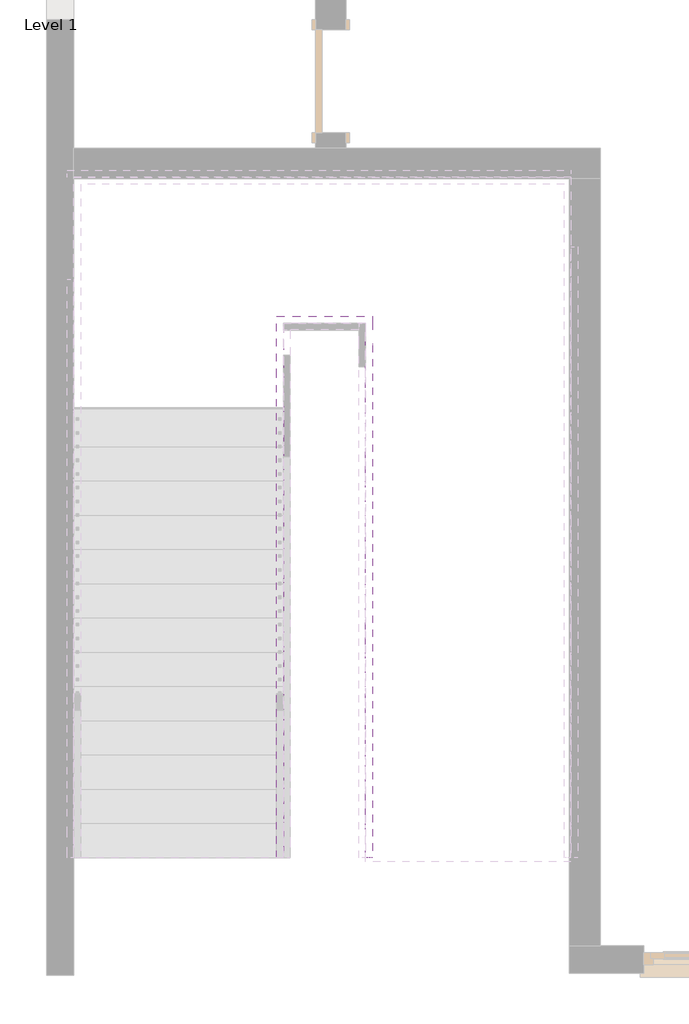
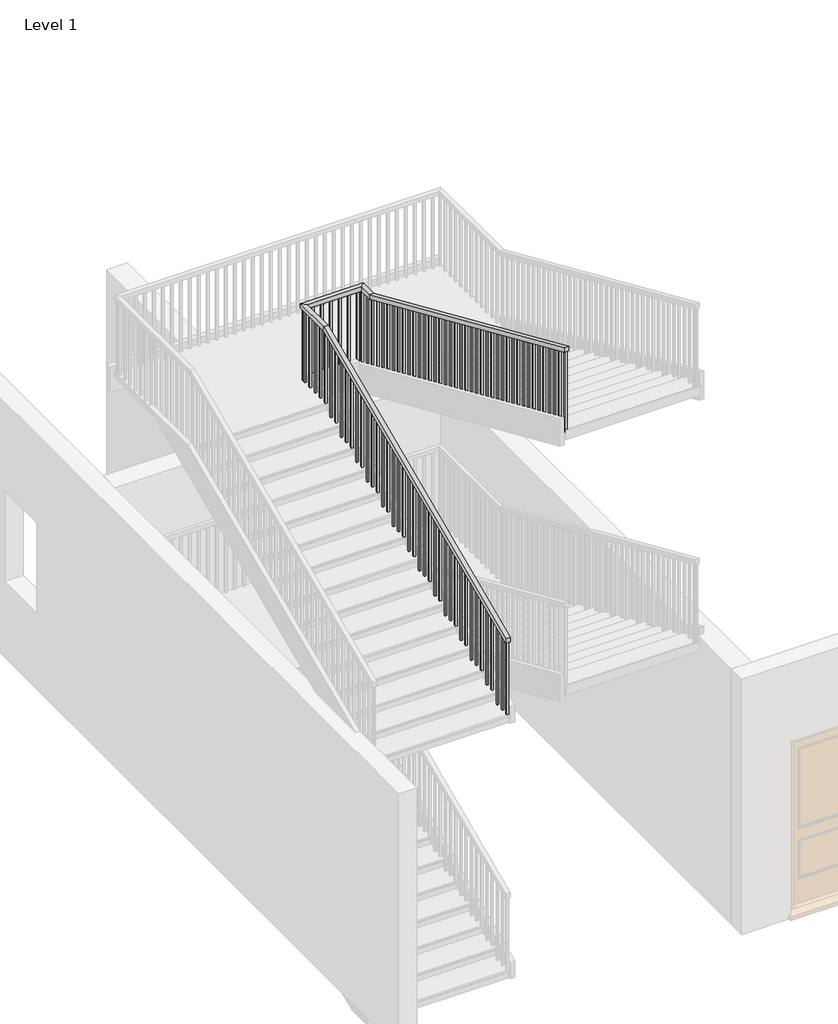
# One storey, part 4 of 6: 1 railing.
"""IFC4 building model written with IfcOpenShell, lengths in millimetres."""

from ifc_helpers import new_model, si_unit, frame, origin, place, context, project, spatial, polyline, outline, extrude, faceted_brep, element, save

model = new_model("IFC4")

# Units and contexts
model_context = context("Model", 3, world=origin())
ifc_project = project(units=[si_unit("LENGTHUNIT", "METRE", prefix="MILLI")], contexts=[model_context])

# Site, building, storey
site = spatial("IfcSite", under=ifc_project)
building = spatial("IfcBuilding", under=site)
storey = spatial("IfcBuildingStorey", under=building, Name="Level 1", Elevation=0.0)

# Railing
placement = place(None, origin())
element("IfcRailing", 1, ObjectType="Handrail - Rectangular", at=placement, inside=storey, context=model_context, shape_type="SolidModel", body=[
    faceted_brep([(-6050.7290366, -6973.0610642, 3769.36), (-6050.7290366, -6973.0610642, 3713.8599828), (-5999.9290366, -6973.0610642, 3713.8599828), (-5999.9290366, -6973.0610642, 3769.36), (-6050.7290366, -3417.0610642, 5334.0), (-6050.7290366, -3406.3792071, 5283.2), (-5999.9290366, -3406.3792071, 5283.2), (-5999.9290366, -3417.0610642, 5334.0), (-6050.7290366, -2959.8610642, 5334.0), (-6050.7290366, -2959.8610642, 5283.2), (-5999.9290366, -3010.6610642, 5283.2), (-5999.9290366, -3010.6610642, 5334.0), (-5339.5290366, -2959.8610642, 5334.0), (-5339.5290366, -2959.8610642, 5283.2), (-5390.3290366, -3010.6610642, 5283.2), (-5390.3290366, -3010.6610642, 5334.0), (-5339.5290366, -3163.0610642, 5334.0), (-5339.5290366, -3173.7429214, 5283.2), (-5390.3290366, -3173.7429214, 5283.2), (-5390.3290366, -3163.0610642, 5334.0), (-5339.5290366, -6973.0610642, 7010.4), (-5390.3290366, -6973.0610642, 7010.4), (-5390.3290366, -6973.0610642, 6954.8999828), (-5339.5290366, -6973.0610642, 6954.8999828)], [[[0, 1, 2, 3]], [[1, 0, 4, 5]], [[2, 1, 5, 6]], [[3, 2, 6, 7]], [[0, 3, 7, 4]], [[5, 4, 8, 9]], [[6, 5, 9, 10]], [[7, 6, 10, 11]], [[4, 7, 11, 8]], [[9, 8, 12, 13]], [[10, 9, 13, 14]], [[11, 10, 14, 15]], [[8, 11, 15, 12]], [[13, 12, 16, 17]], [[14, 13, 17, 18]], [[15, 14, 18, 19]], [[12, 15, 19, 16]], [[20, 21, 22, 23]], [[17, 16, 20, 23]], [[18, 17, 23, 22]], [[19, 18, 22, 21]], [[16, 19, 21, 20]]]),
    extrude(outline(polyline([(-6957.1860642, 6947.9149828), (-6938.1360642, 6939.5329828), (-6938.1360642, 5984.24), (-6957.1860642, 5984.24), (-6957.1860642, 6947.9149828)])), frame((-5374.4540366, 0.0, 0.0), z_axis=(1.0, 0.0, 0.0), x_axis=(0.0, 1.0, 0.0)), (0.0, 0.0, 1.0), 19.05),
    extrude(outline(polyline([(-6855.5860642, 6903.2109828), (-6836.5360642, 6894.8289828), (-6836.5360642, 5984.24), (-6855.5860642, 5984.24), (-6855.5860642, 6903.2109828)])), frame((-5374.4540366, 0.0, 0.0), z_axis=(1.0, 0.0, 0.0), x_axis=(0.0, 1.0, 0.0)), (0.0, 0.0, 1.0), 19.05),
    extrude(outline(polyline([(-6753.9860642, 6858.5069828), (-6734.9360642, 6850.1249828), (-6734.9360642, 5984.24), (-6753.9860642, 5984.24), (-6753.9860642, 6858.5069828)])), frame((-5374.4540366, 0.0, 0.0), z_axis=(1.0, 0.0, 0.0), x_axis=(0.0, 1.0, 0.0)), (0.0, 0.0, 1.0), 19.05),
    extrude(outline(polyline([(-6652.3860642, 6813.8029828), (-6633.3360642, 6805.4209828), (-6633.3360642, 5872.48), (-6652.3860642, 5872.48), (-6652.3860642, 6813.8029828)])), frame((-5374.4540366, 0.0, 0.0), z_axis=(1.0, 0.0, 0.0), x_axis=(0.0, 1.0, 0.0)), (0.0, 0.0, 1.0), 19.05),
    extrude(outline(polyline([(-6550.7860642, 6769.0989828), (-6531.7360642, 6760.7169828), (-6531.7360642, 5872.48), (-6550.7860642, 5872.48), (-6550.7860642, 6769.0989828)])), frame((-5374.4540366, 0.0, 0.0), z_axis=(1.0, 0.0, 0.0), x_axis=(0.0, 1.0, 0.0)), (0.0, 0.0, 1.0), 19.05),
    extrude(outline(polyline([(-6449.1860642, 6724.3949828), (-6430.1360642, 6716.0129828), (-6430.1360642, 5760.72), (-6449.1860642, 5760.72), (-6449.1860642, 6724.3949828)])), frame((-5374.4540366, 0.0, 0.0), z_axis=(1.0, 0.0, 0.0), x_axis=(0.0, 1.0, 0.0)), (0.0, 0.0, 1.0), 19.05),
    extrude(outline(polyline([(-6347.5860642, 6679.6909828), (-6328.5360642, 6671.3089828), (-6328.5360642, 5760.72), (-6347.5860642, 5760.72), (-6347.5860642, 6679.6909828)])), frame((-5374.4540366, 0.0, 0.0), z_axis=(1.0, 0.0, 0.0), x_axis=(0.0, 1.0, 0.0)), (0.0, 0.0, 1.0), 19.05),
    extrude(outline(polyline([(-6245.9860642, 6634.9869828), (-6226.9360642, 6626.6049828), (-6226.9360642, 5760.72), (-6245.9860642, 5760.72), (-6245.9860642, 6634.9869828)])), frame((-5374.4540366, 0.0, 0.0), z_axis=(1.0, 0.0, 0.0), x_axis=(0.0, 1.0, 0.0)), (0.0, 0.0, 1.0), 19.05),
    extrude(outline(polyline([(-6144.3860642, 6590.2829828), (-6125.3360642, 6581.9009828), (-6125.3360642, 5648.96), (-6144.3860642, 5648.96), (-6144.3860642, 6590.2829828)])), frame((-5374.4540366, 0.0, 0.0), z_axis=(1.0, 0.0, 0.0), x_axis=(0.0, 1.0, 0.0)), (0.0, 0.0, 1.0), 19.05),
    extrude(outline(polyline([(-6042.7860642, 6545.5789828), (-6023.7360642, 6537.1969828), (-6023.7360642, 5648.96), (-6042.7860642, 5648.96), (-6042.7860642, 6545.5789828)])), frame((-5374.4540366, 0.0, 0.0), z_axis=(1.0, 0.0, 0.0), x_axis=(0.0, 1.0, 0.0)), (0.0, 0.0, 1.0), 19.05),
    extrude(outline(polyline([(-5941.1860642, 6500.8749828), (-5922.1360642, 6492.4929828), (-5922.1360642, 5537.2), (-5941.1860642, 5537.2), (-5941.1860642, 6500.8749828)])), frame((-5374.4540366, 0.0, 0.0), z_axis=(1.0, 0.0, 0.0), x_axis=(0.0, 1.0, 0.0)), (0.0, 0.0, 1.0), 19.05),
    extrude(outline(polyline([(-5839.5860642, 6456.1709828), (-5820.5360642, 6447.7889828), (-5820.5360642, 5537.2), (-5839.5860642, 5537.2), (-5839.5860642, 6456.1709828)])), frame((-5374.4540366, 0.0, 0.0), z_axis=(1.0, 0.0, 0.0), x_axis=(0.0, 1.0, 0.0)), (0.0, 0.0, 1.0), 19.05),
    extrude(outline(polyline([(-5737.9860642, 6411.4669828), (-5718.9360642, 6403.0849828), (-5718.9360642, 5537.2), (-5737.9860642, 5537.2), (-5737.9860642, 6411.4669828)])), frame((-5374.4540366, 0.0, 0.0), z_axis=(1.0, 0.0, 0.0), x_axis=(0.0, 1.0, 0.0)), (0.0, 0.0, 1.0), 19.05),
    extrude(outline(polyline([(-5636.3860642, 6366.7629828), (-5617.3360642, 6358.3809828), (-5617.3360642, 5425.44), (-5636.3860642, 5425.44), (-5636.3860642, 6366.7629828)])), frame((-5374.4540366, 0.0, 0.0), z_axis=(1.0, 0.0, 0.0), x_axis=(0.0, 1.0, 0.0)), (0.0, 0.0, 1.0), 19.05),
    extrude(outline(polyline([(-5534.7860642, 6322.0589828), (-5515.7360642, 6313.6769828), (-5515.7360642, 5425.44), (-5534.7860642, 5425.44), (-5534.7860642, 6322.0589828)])), frame((-5374.4540366, 0.0, 0.0), z_axis=(1.0, 0.0, 0.0), x_axis=(0.0, 1.0, 0.0)), (0.0, 0.0, 1.0), 19.05),
    extrude(outline(polyline([(-5433.1860642, 6277.3549828), (-5414.1360642, 6268.9729828), (-5414.1360642, 5313.68), (-5433.1860642, 5313.68), (-5433.1860642, 6277.3549828)])), frame((-5374.4540366, 0.0, 0.0), z_axis=(1.0, 0.0, 0.0), x_axis=(0.0, 1.0, 0.0)), (0.0, 0.0, 1.0), 19.05),
    extrude(outline(polyline([(-5331.5860642, 6232.6509828), (-5312.5360642, 6224.2689828), (-5312.5360642, 5313.68), (-5331.5860642, 5313.68), (-5331.5860642, 6232.6509828)])), frame((-5374.4540366, 0.0, 0.0), z_axis=(1.0, 0.0, 0.0), x_axis=(0.0, 1.0, 0.0)), (0.0, 0.0, 1.0), 19.05),
    extrude(outline(polyline([(-5229.9860642, 6187.9469828), (-5210.9360642, 6179.5649828), (-5210.9360642, 5313.68), (-5229.9860642, 5313.68), (-5229.9860642, 6187.9469828)])), frame((-5374.4540366, 0.0, 0.0), z_axis=(1.0, 0.0, 0.0), x_axis=(0.0, 1.0, 0.0)), (0.0, 0.0, 1.0), 19.05),
    extrude(outline(polyline([(-5128.3860642, 6143.2429828), (-5109.3360642, 6134.8609828), (-5109.3360642, 5201.92), (-5128.3860642, 5201.92), (-5128.3860642, 6143.2429828)])), frame((-5374.4540366, 0.0, 0.0), z_axis=(1.0, 0.0, 0.0), x_axis=(0.0, 1.0, 0.0)), (0.0, 0.0, 1.0), 19.05),
    extrude(outline(polyline([(-5026.7860642, 6098.5389828), (-5007.7360642, 6090.1569828), (-5007.7360642, 5201.92), (-5026.7860642, 5201.92), (-5026.7860642, 6098.5389828)])), frame((-5374.4540366, 0.0, 0.0), z_axis=(1.0, 0.0, 0.0), x_axis=(0.0, 1.0, 0.0)), (0.0, 0.0, 1.0), 19.05),
    extrude(outline(polyline([(-4925.1860642, 6053.8349828), (-4906.1360642, 6045.4529828), (-4906.1360642, 5090.16), (-4925.1860642, 5090.16), (-4925.1860642, 6053.8349828)])), frame((-5374.4540366, 0.0, 0.0), z_axis=(1.0, 0.0, 0.0), x_axis=(0.0, 1.0, 0.0)), (0.0, 0.0, 1.0), 19.05),
    extrude(outline(polyline([(-4823.5860642, 6009.1309828), (-4804.5360642, 6000.7489828), (-4804.5360642, 5090.16), (-4823.5860642, 5090.16), (-4823.5860642, 6009.1309828)])), frame((-5374.4540366, 0.0, 0.0), z_axis=(1.0, 0.0, 0.0), x_axis=(0.0, 1.0, 0.0)), (0.0, 0.0, 1.0), 19.05),
    extrude(outline(polyline([(-4721.9860642, 5964.4269828), (-4702.9360642, 5956.0449828), (-4702.9360642, 5090.16), (-4721.9860642, 5090.16), (-4721.9860642, 5964.4269828)])), frame((-5374.4540366, 0.0, 0.0), z_axis=(1.0, 0.0, 0.0), x_axis=(0.0, 1.0, 0.0)), (0.0, 0.0, 1.0), 19.05),
    extrude(outline(polyline([(-4620.3860642, 5919.7229828), (-4601.3360642, 5911.3409828), (-4601.3360642, 4978.4), (-4620.3860642, 4978.4), (-4620.3860642, 5919.7229828)])), frame((-5374.4540366, 0.0, 0.0), z_axis=(1.0, 0.0, 0.0), x_axis=(0.0, 1.0, 0.0)), (0.0, 0.0, 1.0), 19.05),
    extrude(outline(polyline([(-4518.7860642, 5875.0189828), (-4499.7360642, 5866.6369828), (-4499.7360642, 4978.4), (-4518.7860642, 4978.4), (-4518.7860642, 5875.0189828)])), frame((-5374.4540366, 0.0, 0.0), z_axis=(1.0, 0.0, 0.0), x_axis=(0.0, 1.0, 0.0)), (0.0, 0.0, 1.0), 19.05),
    extrude(outline(polyline([(-4417.1860642, 5830.3149828), (-4398.1360642, 5821.9329828), (-4398.1360642, 4866.64), (-4417.1860642, 4866.64), (-4417.1860642, 5830.3149828)])), frame((-5374.4540366, 0.0, 0.0), z_axis=(1.0, 0.0, 0.0), x_axis=(0.0, 1.0, 0.0)), (0.0, 0.0, 1.0), 19.05),
    extrude(outline(polyline([(-4315.5860642, 5785.6109828), (-4296.5360642, 5777.2289828), (-4296.5360642, 4866.64), (-4315.5860642, 4866.64), (-4315.5860642, 5785.6109828)])), frame((-5374.4540366, 0.0, 0.0), z_axis=(1.0, 0.0, 0.0), x_axis=(0.0, 1.0, 0.0)), (0.0, 0.0, 1.0), 19.05),
    extrude(outline(polyline([(-4213.9860642, 5740.9069828), (-4194.9360642, 5732.5249828), (-4194.9360642, 4866.64), (-4213.9860642, 4866.64), (-4213.9860642, 5740.9069828)])), frame((-5374.4540366, 0.0, 0.0), z_axis=(1.0, 0.0, 0.0), x_axis=(0.0, 1.0, 0.0)), (0.0, 0.0, 1.0), 19.05),
    extrude(outline(polyline([(-4112.3860642, 5696.2029828), (-4093.3360642, 5687.8209828), (-4093.3360642, 4754.88), (-4112.3860642, 4754.88), (-4112.3860642, 5696.2029828)])), frame((-5374.4540366, 0.0, 0.0), z_axis=(1.0, 0.0, 0.0), x_axis=(0.0, 1.0, 0.0)), (0.0, 0.0, 1.0), 19.05),
    extrude(outline(polyline([(-4010.7860642, 5651.4989828), (-3991.7360642, 5643.1169828), (-3991.7360642, 4754.88), (-4010.7860642, 4754.88), (-4010.7860642, 5651.4989828)])), frame((-5374.4540366, 0.0, 0.0), z_axis=(1.0, 0.0, 0.0), x_axis=(0.0, 1.0, 0.0)), (0.0, 0.0, 1.0), 19.05),
    extrude(outline(polyline([(-3909.1860642, 5606.7949828), (-3890.1360642, 5598.4129828), (-3890.1360642, 4643.12), (-3909.1860642, 4643.12), (-3909.1860642, 5606.7949828)])), frame((-5374.4540366, 0.0, 0.0), z_axis=(1.0, 0.0, 0.0), x_axis=(0.0, 1.0, 0.0)), (0.0, 0.0, 1.0), 19.05),
    extrude(outline(polyline([(-3807.5860642, 5562.0909828), (-3788.5360642, 5553.7089828), (-3788.5360642, 4643.12), (-3807.5860642, 4643.12), (-3807.5860642, 5562.0909828)])), frame((-5374.4540366, 0.0, 0.0), z_axis=(1.0, 0.0, 0.0), x_axis=(0.0, 1.0, 0.0)), (0.0, 0.0, 1.0), 19.05),
    extrude(outline(polyline([(-3705.9860642, 5517.3869828), (-3686.9360642, 5509.0049828), (-3686.9360642, 4643.12), (-3705.9860642, 4643.12), (-3705.9860642, 5517.3869828)])), frame((-5374.4540366, 0.0, 0.0), z_axis=(1.0, 0.0, 0.0), x_axis=(0.0, 1.0, 0.0)), (0.0, 0.0, 1.0), 19.05),
    extrude(outline(polyline([(-3604.3860642, 5472.6829828), (-3585.3360642, 5464.3009828), (-3585.3360642, 4531.36), (-3604.3860642, 4531.36), (-3604.3860642, 5472.6829828)])), frame((-5374.4540366, 0.0, 0.0), z_axis=(1.0, 0.0, 0.0), x_axis=(0.0, 1.0, 0.0)), (0.0, 0.0, 1.0), 19.05),
    extrude(outline(polyline([(-3502.7860642, 5427.9789828), (-3483.7360642, 5419.5969828), (-3483.7360642, 4531.36), (-3502.7860642, 4531.36), (-3502.7860642, 5427.9789828)])), frame((-5374.4540366, 0.0, 0.0), z_axis=(1.0, 0.0, 0.0), x_axis=(0.0, 1.0, 0.0)), (0.0, 0.0, 1.0), 19.05),
    extrude(outline(polyline([(-3401.1860642, 5383.2749828), (-3382.1360642, 5374.8929828), (-3382.1360642, 4419.6), (-3401.1860642, 4419.6), (-3401.1860642, 5383.2749828)])), frame((-5374.4540366, 0.0, 0.0), z_axis=(1.0, 0.0, 0.0), x_axis=(0.0, 1.0, 0.0)), (0.0, 0.0, 1.0), 19.05),
    extrude(outline(polyline([(-3299.5860642, 5338.5709828), (-3280.5360642, 5330.1889828), (-3280.5360642, 4419.6), (-3299.5860642, 4419.6), (-3299.5860642, 5338.5709828)])), frame((-5374.4540366, 0.0, 0.0), z_axis=(1.0, 0.0, 0.0), x_axis=(0.0, 1.0, 0.0)), (0.0, 0.0, 1.0), 19.05),
    extrude(outline(polyline([(-3197.9860642, 5293.8669828), (-3178.9360642, 5285.4849828), (-3178.9360642, 4419.6), (-3197.9860642, 4419.6), (-3197.9860642, 5293.8669828)])), frame((-5374.4540366, 0.0, 0.0), z_axis=(1.0, 0.0, 0.0), x_axis=(0.0, 1.0, 0.0)), (0.0, 0.0, 1.0), 19.05),
    extrude(outline(polyline([(-5374.4540366, -3077.3360642), (-5355.4040366, -3077.3360642), (-5355.4040366, -3096.3860642), (-5374.4540366, -3096.3860642), (-5374.4540366, -3077.3360642)])), frame((0.0, 0.0, 4419.6), z_axis=(0.0, 0.0, 1.0), x_axis=(1.0, 0.0, 0.0)), (0.0, 0.0, 1.0), 863.6),
    extrude(outline(polyline([(-5425.2540366, -2994.7860642), (-5425.2540366, -2975.7360642), (-5406.2040366, -2975.7360642), (-5406.2040366, -2994.7860642), (-5425.2540366, -2994.7860642)])), frame((0.0, 0.0, 4419.6), z_axis=(0.0, 0.0, 1.0), x_axis=(1.0, 0.0, 0.0)), (0.0, 0.0, 1.0), 863.6),
    extrude(outline(polyline([(-5526.8540366, -2994.7860642), (-5526.8540366, -2975.7360642), (-5507.8040366, -2975.7360642), (-5507.8040366, -2994.7860642), (-5526.8540366, -2994.7860642)])), frame((0.0, 0.0, 4419.6), z_axis=(0.0, 0.0, 1.0), x_axis=(1.0, 0.0, 0.0)), (0.0, 0.0, 1.0), 863.6),
    extrude(outline(polyline([(-5628.4540366, -2994.7860642), (-5628.4540366, -2975.7360642), (-5609.4040366, -2975.7360642), (-5609.4040366, -2994.7860642), (-5628.4540366, -2994.7860642)])), frame((0.0, 0.0, 4419.6), z_axis=(0.0, 0.0, 1.0), x_axis=(1.0, 0.0, 0.0)), (0.0, 0.0, 1.0), 863.6),
    extrude(outline(polyline([(-5730.0540366, -2994.7860642), (-5730.0540366, -2975.7360642), (-5711.0040366, -2975.7360642), (-5711.0040366, -2994.7860642), (-5730.0540366, -2994.7860642)])), frame((0.0, 0.0, 4419.6), z_axis=(0.0, 0.0, 1.0), x_axis=(1.0, 0.0, 0.0)), (0.0, 0.0, 1.0), 863.6),
    extrude(outline(polyline([(-5831.6540366, -2994.7860642), (-5831.6540366, -2975.7360642), (-5812.6040366, -2975.7360642), (-5812.6040366, -2994.7860642), (-5831.6540366, -2994.7860642)])), frame((0.0, 0.0, 4419.6), z_axis=(0.0, 0.0, 1.0), x_axis=(1.0, 0.0, 0.0)), (0.0, 0.0, 1.0), 863.6),
    extrude(outline(polyline([(-5933.2540366, -2994.7860642), (-5933.2540366, -2975.7360642), (-5914.2040366, -2975.7360642), (-5914.2040366, -2994.7860642), (-5933.2540366, -2994.7860642)])), frame((0.0, 0.0, 4419.6), z_axis=(0.0, 0.0, 1.0), x_axis=(1.0, 0.0, 0.0)), (0.0, 0.0, 1.0), 863.6),
    extrude(outline(polyline([(-6015.8040366, -3020.1860642), (-6034.8540366, -3020.1860642), (-6034.8540366, -3001.1360642), (-6015.8040366, -3001.1360642), (-6015.8040366, -3020.1860642)])), frame((0.0, 0.0, 4419.6), z_axis=(0.0, 0.0, 1.0), x_axis=(1.0, 0.0, 0.0)), (0.0, 0.0, 1.0), 863.6),
    extrude(outline(polyline([(-6015.8040366, -3121.7860642), (-6034.8540366, -3121.7860642), (-6034.8540366, -3102.7360642), (-6015.8040366, -3102.7360642), (-6015.8040366, -3121.7860642)])), frame((0.0, 0.0, 4419.6), z_axis=(0.0, 0.0, 1.0), x_axis=(1.0, 0.0, 0.0)), (0.0, 0.0, 1.0), 863.6),
    extrude(outline(polyline([(-6015.8040366, -3223.3860642), (-6034.8540366, -3223.3860642), (-6034.8540366, -3204.3360642), (-6015.8040366, -3204.3360642), (-6015.8040366, -3223.3860642)])), frame((0.0, 0.0, 4419.6), z_axis=(0.0, 0.0, 1.0), x_axis=(1.0, 0.0, 0.0)), (0.0, 0.0, 1.0), 863.6),
    extrude(outline(polyline([(-6015.8040366, -3324.9860642), (-6034.8540366, -3324.9860642), (-6034.8540366, -3305.9360642), (-6015.8040366, -3305.9360642), (-6015.8040366, -3324.9860642)])), frame((0.0, 0.0, 4419.6), z_axis=(0.0, 0.0, 1.0), x_axis=(1.0, 0.0, 0.0)), (0.0, 0.0, 1.0), 863.6),
    extrude(outline(polyline([(-3426.5860642, 5274.3089828), (-3407.5360642, 5282.6909828), (-3407.5360642, 4419.6), (-3426.5860642, 4419.6), (-3426.5860642, 5274.3089828)])), frame((-6034.8540366, 0.0, 0.0), z_axis=(1.0, 0.0, 0.0), x_axis=(0.0, 1.0, 0.0)), (0.0, 0.0, 1.0), 19.05),
    extrude(outline(polyline([(-3528.1860642, 5229.6049828), (-3509.1360642, 5237.9869828), (-3509.1360642, 4307.84), (-3528.1860642, 4307.84), (-3528.1860642, 5229.6049828)])), frame((-6034.8540366, 0.0, 0.0), z_axis=(1.0, 0.0, 0.0), x_axis=(0.0, 1.0, 0.0)), (0.0, 0.0, 1.0), 19.05),
    extrude(outline(polyline([(-3629.7860642, 5184.9009828), (-3610.7360642, 5193.2829828), (-3610.7360642, 4307.84), (-3629.7860642, 4307.84), (-3629.7860642, 5184.9009828)])), frame((-6034.8540366, 0.0, 0.0), z_axis=(1.0, 0.0, 0.0), x_axis=(0.0, 1.0, 0.0)), (0.0, 0.0, 1.0), 19.05),
    extrude(outline(polyline([(-3731.3860642, 5140.1969828), (-3712.3360642, 5148.5789828), (-3712.3360642, 4196.08), (-3731.3860642, 4196.08), (-3731.3860642, 5140.1969828)])), frame((-6034.8540366, 0.0, 0.0), z_axis=(1.0, 0.0, 0.0), x_axis=(0.0, 1.0, 0.0)), (0.0, 0.0, 1.0), 19.05),
    extrude(outline(polyline([(-3832.9860642, 5095.4929828), (-3813.9360642, 5103.8749828), (-3813.9360642, 4196.08), (-3832.9860642, 4196.08), (-3832.9860642, 5095.4929828)])), frame((-6034.8540366, 0.0, 0.0), z_axis=(1.0, 0.0, 0.0), x_axis=(0.0, 1.0, 0.0)), (0.0, 0.0, 1.0), 19.05),
    extrude(outline(polyline([(-3934.5860642, 5050.7889828), (-3915.5360642, 5059.1709828), (-3915.5360642, 4196.08), (-3934.5860642, 4196.08), (-3934.5860642, 5050.7889828)])), frame((-6034.8540366, 0.0, 0.0), z_axis=(1.0, 0.0, 0.0), x_axis=(0.0, 1.0, 0.0)), (0.0, 0.0, 1.0), 19.05),
    extrude(outline(polyline([(-4036.1860642, 5006.0849828), (-4017.1360642, 5014.4669828), (-4017.1360642, 4084.32), (-4036.1860642, 4084.32), (-4036.1860642, 5006.0849828)])), frame((-6034.8540366, 0.0, 0.0), z_axis=(1.0, 0.0, 0.0), x_axis=(0.0, 1.0, 0.0)), (0.0, 0.0, 1.0), 19.05),
    extrude(outline(polyline([(-4137.7860642, 4961.3809828), (-4118.7360642, 4969.7629828), (-4118.7360642, 4084.32), (-4137.7860642, 4084.32), (-4137.7860642, 4961.3809828)])), frame((-6034.8540366, 0.0, 0.0), z_axis=(1.0, 0.0, 0.0), x_axis=(0.0, 1.0, 0.0)), (0.0, 0.0, 1.0), 19.05),
    extrude(outline(polyline([(-4239.3860642, 4916.6769828), (-4220.3360642, 4925.0589828), (-4220.3360642, 3972.56), (-4239.3860642, 3972.56), (-4239.3860642, 4916.6769828)])), frame((-6034.8540366, 0.0, 0.0), z_axis=(1.0, 0.0, 0.0), x_axis=(0.0, 1.0, 0.0)), (0.0, 0.0, 1.0), 19.05),
    extrude(outline(polyline([(-4340.9860642, 4871.9729828), (-4321.9360642, 4880.3549828), (-4321.9360642, 3972.56), (-4340.9860642, 3972.56), (-4340.9860642, 4871.9729828)])), frame((-6034.8540366, 0.0, 0.0), z_axis=(1.0, 0.0, 0.0), x_axis=(0.0, 1.0, 0.0)), (0.0, 0.0, 1.0), 19.05),
    extrude(outline(polyline([(-4442.5860642, 4827.2689828), (-4423.5360642, 4835.6509828), (-4423.5360642, 3972.56), (-4442.5860642, 3972.56), (-4442.5860642, 4827.2689828)])), frame((-6034.8540366, 0.0, 0.0), z_axis=(1.0, 0.0, 0.0), x_axis=(0.0, 1.0, 0.0)), (0.0, 0.0, 1.0), 19.05),
    extrude(outline(polyline([(-4544.1860642, 4782.5649828), (-4525.1360642, 4790.9469828), (-4525.1360642, 3860.8), (-4544.1860642, 3860.8), (-4544.1860642, 4782.5649828)])), frame((-6034.8540366, 0.0, 0.0), z_axis=(1.0, 0.0, 0.0), x_axis=(0.0, 1.0, 0.0)), (0.0, 0.0, 1.0), 19.05),
    extrude(outline(polyline([(-4645.7860642, 4737.8609828), (-4626.7360642, 4746.2429828), (-4626.7360642, 3860.8), (-4645.7860642, 3860.8), (-4645.7860642, 4737.8609828)])), frame((-6034.8540366, 0.0, 0.0), z_axis=(1.0, 0.0, 0.0), x_axis=(0.0, 1.0, 0.0)), (0.0, 0.0, 1.0), 19.05),
    extrude(outline(polyline([(-4747.3860642, 4693.1569828), (-4728.3360642, 4701.5389828), (-4728.3360642, 3749.04), (-4747.3860642, 3749.04), (-4747.3860642, 4693.1569828)])), frame((-6034.8540366, 0.0, 0.0), z_axis=(1.0, 0.0, 0.0), x_axis=(0.0, 1.0, 0.0)), (0.0, 0.0, 1.0), 19.05),
    extrude(outline(polyline([(-4848.9860642, 4648.4529828), (-4829.9360642, 4656.8349828), (-4829.9360642, 3749.04), (-4848.9860642, 3749.04), (-4848.9860642, 4648.4529828)])), frame((-6034.8540366, 0.0, 0.0), z_axis=(1.0, 0.0, 0.0), x_axis=(0.0, 1.0, 0.0)), (0.0, 0.0, 1.0), 19.05),
    extrude(outline(polyline([(-4950.5860642, 4603.7489828), (-4931.5360642, 4612.1309828), (-4931.5360642, 3749.04), (-4950.5860642, 3749.04), (-4950.5860642, 4603.7489828)])), frame((-6034.8540366, 0.0, 0.0), z_axis=(1.0, 0.0, 0.0), x_axis=(0.0, 1.0, 0.0)), (0.0, 0.0, 1.0), 19.05),
    extrude(outline(polyline([(-5052.1860642, 4559.0449828), (-5033.1360642, 4567.4269828), (-5033.1360642, 3637.28), (-5052.1860642, 3637.28), (-5052.1860642, 4559.0449828)])), frame((-6034.8540366, 0.0, 0.0), z_axis=(1.0, 0.0, 0.0), x_axis=(0.0, 1.0, 0.0)), (0.0, 0.0, 1.0), 19.05),
    extrude(outline(polyline([(-5153.7860642, 4514.3409828), (-5134.7360642, 4522.7229828), (-5134.7360642, 3637.28), (-5153.7860642, 3637.28), (-5153.7860642, 4514.3409828)])), frame((-6034.8540366, 0.0, 0.0), z_axis=(1.0, 0.0, 0.0), x_axis=(0.0, 1.0, 0.0)), (0.0, 0.0, 1.0), 19.05),
    extrude(outline(polyline([(-5255.3860642, 4469.6369828), (-5236.3360642, 4478.0189828), (-5236.3360642, 3525.52), (-5255.3860642, 3525.52), (-5255.3860642, 4469.6369828)])), frame((-6034.8540366, 0.0, 0.0), z_axis=(1.0, 0.0, 0.0), x_axis=(0.0, 1.0, 0.0)), (0.0, 0.0, 1.0), 19.05),
    extrude(outline(polyline([(-5356.9860642, 4424.9329828), (-5337.9360642, 4433.3149828), (-5337.9360642, 3525.52), (-5356.9860642, 3525.52), (-5356.9860642, 4424.9329828)])), frame((-6034.8540366, 0.0, 0.0), z_axis=(1.0, 0.0, 0.0), x_axis=(0.0, 1.0, 0.0)), (0.0, 0.0, 1.0), 19.05),
    extrude(outline(polyline([(-5458.5860642, 4380.2289828), (-5439.5360642, 4388.6109828), (-5439.5360642, 3525.52), (-5458.5860642, 3525.52), (-5458.5860642, 4380.2289828)])), frame((-6034.8540366, 0.0, 0.0), z_axis=(1.0, 0.0, 0.0), x_axis=(0.0, 1.0, 0.0)), (0.0, 0.0, 1.0), 19.05),
    extrude(outline(polyline([(-5560.1860642, 4335.5249828), (-5541.1360642, 4343.9069828), (-5541.1360642, 3413.76), (-5560.1860642, 3413.76), (-5560.1860642, 4335.5249828)])), frame((-6034.8540366, 0.0, 0.0), z_axis=(1.0, 0.0, 0.0), x_axis=(0.0, 1.0, 0.0)), (0.0, 0.0, 1.0), 19.05),
    extrude(outline(polyline([(-5661.7860642, 4290.8209828), (-5642.7360642, 4299.2029828), (-5642.7360642, 3413.76), (-5661.7860642, 3413.76), (-5661.7860642, 4290.8209828)])), frame((-6034.8540366, 0.0, 0.0), z_axis=(1.0, 0.0, 0.0), x_axis=(0.0, 1.0, 0.0)), (0.0, 0.0, 1.0), 19.05),
    extrude(outline(polyline([(-5763.3860642, 4246.1169828), (-5744.3360642, 4254.4989828), (-5744.3360642, 3302.0), (-5763.3860642, 3302.0), (-5763.3860642, 4246.1169828)])), frame((-6034.8540366, 0.0, 0.0), z_axis=(1.0, 0.0, 0.0), x_axis=(0.0, 1.0, 0.0)), (0.0, 0.0, 1.0), 19.05),
    extrude(outline(polyline([(-5864.9860642, 4201.4129828), (-5845.9360642, 4209.7949828), (-5845.9360642, 3302.0), (-5864.9860642, 3302.0), (-5864.9860642, 4201.4129828)])), frame((-6034.8540366, 0.0, 0.0), z_axis=(1.0, 0.0, 0.0), x_axis=(0.0, 1.0, 0.0)), (0.0, 0.0, 1.0), 19.05),
    extrude(outline(polyline([(-5966.5860642, 4156.7089828), (-5947.5360642, 4165.0909828), (-5947.5360642, 3302.0), (-5966.5860642, 3302.0), (-5966.5860642, 4156.7089828)])), frame((-6034.8540366, 0.0, 0.0), z_axis=(1.0, 0.0, 0.0), x_axis=(0.0, 1.0, 0.0)), (0.0, 0.0, 1.0), 19.05),
    extrude(outline(polyline([(-6068.1860642, 4112.0049828), (-6049.1360642, 4120.3869828), (-6049.1360642, 3190.24), (-6068.1860642, 3190.24), (-6068.1860642, 4112.0049828)])), frame((-6034.8540366, 0.0, 0.0), z_axis=(1.0, 0.0, 0.0), x_axis=(0.0, 1.0, 0.0)), (0.0, 0.0, 1.0), 19.05),
    extrude(outline(polyline([(-6169.7860642, 4067.3009828), (-6150.7360642, 4075.6829828), (-6150.7360642, 3190.24), (-6169.7860642, 3190.24), (-6169.7860642, 4067.3009828)])), frame((-6034.8540366, 0.0, 0.0), z_axis=(1.0, 0.0, 0.0), x_axis=(0.0, 1.0, 0.0)), (0.0, 0.0, 1.0), 19.05),
    extrude(outline(polyline([(-6271.3860642, 4022.5969828), (-6252.3360642, 4030.9789828), (-6252.3360642, 3078.48), (-6271.3860642, 3078.48), (-6271.3860642, 4022.5969828)])), frame((-6034.8540366, 0.0, 0.0), z_axis=(1.0, 0.0, 0.0), x_axis=(0.0, 1.0, 0.0)), (0.0, 0.0, 1.0), 19.05),
    extrude(outline(polyline([(-6372.9860642, 3977.8929828), (-6353.9360642, 3986.2749828), (-6353.9360642, 3078.48), (-6372.9860642, 3078.48), (-6372.9860642, 3977.8929828)])), frame((-6034.8540366, 0.0, 0.0), z_axis=(1.0, 0.0, 0.0), x_axis=(0.0, 1.0, 0.0)), (0.0, 0.0, 1.0), 19.05),
    extrude(outline(polyline([(-6474.5860642, 3933.1889828), (-6455.5360642, 3941.5709828), (-6455.5360642, 3078.48), (-6474.5860642, 3078.48), (-6474.5860642, 3933.1889828)])), frame((-6034.8540366, 0.0, 0.0), z_axis=(1.0, 0.0, 0.0), x_axis=(0.0, 1.0, 0.0)), (0.0, 0.0, 1.0), 19.05),
    extrude(outline(polyline([(-6576.1860642, 3888.4849828), (-6557.1360642, 3896.8669828), (-6557.1360642, 2966.72), (-6576.1860642, 2966.72), (-6576.1860642, 3888.4849828)])), frame((-6034.8540366, 0.0, 0.0), z_axis=(1.0, 0.0, 0.0), x_axis=(0.0, 1.0, 0.0)), (0.0, 0.0, 1.0), 19.05),
    extrude(outline(polyline([(-6677.7860642, 3843.7809828), (-6658.7360642, 3852.1629828), (-6658.7360642, 2966.72), (-6677.7860642, 2966.72), (-6677.7860642, 3843.7809828)])), frame((-6034.8540366, 0.0, 0.0), z_axis=(1.0, 0.0, 0.0), x_axis=(0.0, 1.0, 0.0)), (0.0, 0.0, 1.0), 19.05),
    extrude(outline(polyline([(-6779.3860642, 3799.0769828), (-6760.3360642, 3807.4589828), (-6760.3360642, 2854.96), (-6779.3860642, 2854.96), (-6779.3860642, 3799.0769828)])), frame((-6034.8540366, 0.0, 0.0), z_axis=(1.0, 0.0, 0.0), x_axis=(0.0, 1.0, 0.0)), (0.0, 0.0, 1.0), 19.05),
    extrude(outline(polyline([(-6880.9860642, 3754.3729828), (-6861.9360642, 3762.7549828), (-6861.9360642, 2854.96), (-6880.9860642, 2854.96), (-6880.9860642, 3754.3729828)])), frame((-6034.8540366, 0.0, 0.0), z_axis=(1.0, 0.0, 0.0), x_axis=(0.0, 1.0, 0.0)), (0.0, 0.0, 1.0), 19.05),
    extrude(outline(polyline([(-5374.4540366, -2994.7860642), (-5374.4540366, -2975.7360642), (-5355.4040366, -2975.7360642), (-5355.4040366, -2994.7860642), (-5374.4540366, -2994.7860642)])), frame((0.0, 0.0, 4419.6), z_axis=(0.0, 0.0, 1.0), x_axis=(1.0, 0.0, 0.0)), (0.0, 0.0, 1.0), 863.6),
    extrude(outline(polyline([(-6015.8040366, -2994.7860642), (-6034.8540366, -2994.7860642), (-6034.8540366, -2975.7360642), (-6015.8040366, -2975.7360642), (-6015.8040366, -2994.7860642)])), frame((0.0, 0.0, 4419.6), z_axis=(0.0, 0.0, 1.0), x_axis=(1.0, 0.0, 0.0)), (0.0, 0.0, 1.0), 863.6),
    extrude(outline(polyline([(-6973.0610642, 6954.8999828), (-6954.0110642, 6946.5179828), (-6954.0110642, 5984.24), (-6973.0610642, 5984.24), (-6973.0610642, 6954.8999828)])), frame((-5374.4540366, 0.0, 0.0), z_axis=(1.0, 0.0, 0.0), x_axis=(0.0, 1.0, 0.0)), (0.0, 0.0, 1.0), 19.05),
    extrude(outline(polyline([(-6973.0610642, 3713.8599828), (-6954.0110642, 3722.2419828), (-6954.0110642, 2854.96), (-6973.0610642, 2854.96), (-6973.0610642, 3713.8599828)])), frame((-6034.8540366, 0.0, 0.0), z_axis=(1.0, 0.0, 0.0), x_axis=(0.0, 1.0, 0.0)), (0.0, 0.0, 1.0), 19.05),
])

save(model, "model.ifc")

# Revit data of these elements
# Type "Handrail - Rectangular"
#   Assembly Code = "C2010400"
#   built-in parameter 1008612 = 0.0416667 (stored number, unit not read)
#   built-in parameter 1008611 = 0.0416667 (stored number, unit not read)
#   built-in parameter 1008609 = 0.333333 (stored number, unit not read)
#   built-in parameter 1008604 = 0.166667 (stored number, unit not read)
#   built-in parameter 1008603 = 0.166667 (stored number, unit not read)
#   Railing Height = 3' - 0"
#   built-in parameter 1008630 = 2
#   built-in parameter 1008610 = 2
#   built-in parameter 1008618 = Baluster - Square : 3/4"
# Element 1 (IfcRailing, "Handrail - Rectangular")
#   Phase Created = New Construction
